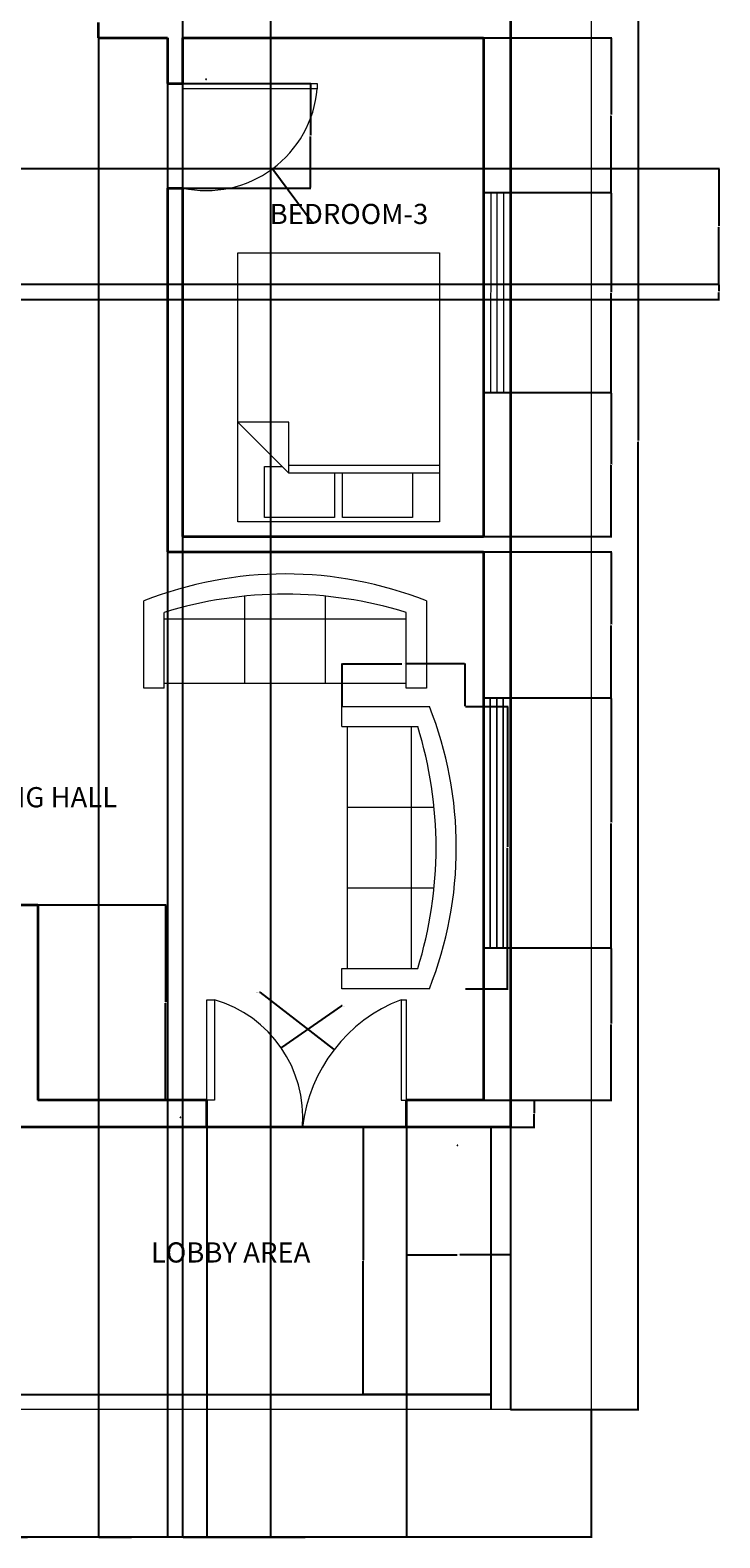
# Model space of a CAD drawing. Units: inches. Extents: x 4700 to 5209, y 8078 to 8754.
# Tile 3 of 5: x 5004 to 5209, y 8078 to 8526. Entities that reach past the tile are written whole.
import ezdxf

# ---------------------------------------------------------------- set-up
doc = ezdxf.new("R2010")
doc.units = ezdxf.units.IN
for name, color, linetype, lineweight in [('A-ANNO-DIMS', 2, 'Continuous', 18), ('A-AREA-IDEN', 7, 'Continuous', 18), ('A-DOOR', 3, 'Continuous', 18), ('A-FLOR', 7, 'Continuous', 25), ('A-FURN', 8, 'Continuous', 18), ('A-GLAZ', 4, 'Continuous', 18), ('A-WALL', 7, 'Continuous', 35), ('C-PROP', 8, 'Continuous', 18)]:
    doc.layers.add(name, color=color, linetype=linetype, lineweight=lineweight)
doc.styles.get("Standard").update_dxf_attribs({"font": 'arial.ttf'})
doc.dimstyles.get("Standard").update_dxf_attribs({"dimtxt": 0.18, "dimasz": 0.18, "dimexe": 0.18, "dimexo": 0.0625, "dimgap": 0.09, "dimtad": 0, "dimtih": 1, "dimtoh": 1, "dimdec": 4, "dimzin": 0, "dimdsep": 46, "dimtxsty": 'Standard', "dimcen": 0.09, "dimadec": 0, "dimazin": 0, "dimtfac": 1, "dimtdec": 4, "dimtofl": 0, "dimtmove": 0, "dimatfit": 3, "dimfxl": 1, "dimtolj": 1, "dimtzin": 0, "dimarcsym": 0})

# ---------------------------------------------------------------- blocks, each defined once
blk = doc.blocks.new('Sofa - Roundback 7 ft.')
for p, q in [((-12.00002, -32.4421), (-12.00003, -6.5971)), ((11.99997, -32.4421), (11.99998, -6.5971)), ((-36.000027, -34), (-36.000027, -11.4696)), ((-35.999844, -13.3819), (35.9998, -13.3819)), ((35.99998, -34), (35.99998, -11.4696)), ((-36.000027, -32.4421), (35.99998, -32.4421))]:
    blk.add_line(p, q)
for points in [[(-36.000027, -34), (-42.000027, -34), (-42.000027, -8)], [(41.99998, -8), (41.99998, -34), (35.99998, -34)]]:
    blk.add_lwpolyline(points)
for centre, radius, start, end in [((0, -114.25), 114.25, 68.43141, 111.5686), ((-0.00001, -127.1968), 121.1968, 72.72033, 107.2797)]:
    blk.add_arc(centre, radius, start, end)
blk = doc.blocks.new('Bed - Queen')
for p, q in [((0, -80.00003), (0, 0)), ((0, 0), (59.99999, 0)), ((59.99999, 0), (59.99999, -80.00003)), ((7.99999, -1.2), (28.79998, -1.2)), ((7.99999, -14.4), (7.99999, -1.2)), ((28.79998, -1.2), (28.79998, -14.4)), ((31.19999, -1.2), (51.99999, -1.2)), ((31.19999, -14.4), (31.19999, -1.2)), ((51.99999, -1.2), (51.99999, -16.4)), ((0, -14.4), (44.8, -14.4)), ((44.8, -16.8), (0, -16.8)), ((59.99999, -29.6), (44.8, -14.4)), ((44.8, -14.4), (44.8, -29.6)), ((51.99999, -16.4), (46.79936, -16.4)), ((44.8, -29.6), (59.99999, -29.6)), ((59.99999, -80.00003), (0, -80.00003))]:
    blk.add_line(p, q)
blk = doc.blocks.new('*D10')
at = {"layer": 'A-ANNO-DIMS', "color": 0, "lineweight": -2, "transparency": 16777216}
for p, q in [((5133.42, 8324.88), (5146.13, 8324.88)), ((5145.95, 8324.7), (5145.95, 8283.06)), ((5145.95, 8241.06), (5145.95, 8282.7)), ((5133.42, 8240.88), (5146.13, 8240.88))]:
    blk.add_line(p, q, dxfattribs=at)
at = {"layer": 'A-ANNO-DIMS', "color": 0, "transparency": 16777216}
for points in [[(5145.92, 8324.7), (5145.98, 8324.7), (5145.95, 8324.88)], [(5145.92, 8241.06), (5145.98, 8241.06), (5145.95, 8240.88)]]:
    blk.add_solid(points, dxfattribs=at)
at = {"layer": 'Defpoints', "color": 0, "transparency": 16777216}
for p in [(5133.35, 8324.88), (5133.35, 8240.88), (5145.95, 8240.88)]:
    blk.add_point(p, dxfattribs=at)
at = {"layer": 'A-ANNO-DIMS', "color": 0, "transparency": 16777216, "insert": (5145.95, 8282.88), "char_height": 0.18, "attachment_point": 5}
blk.add_mtext('\\A1;SOFA 84 TYP.', dxfattribs=at)
blk = doc.blocks.new('*D11')
at = {"layer": 'A-ANNO-DIMS', "color": 0, "lineweight": -2, "transparency": 16777216}
for p, q in [((5096.69, 8324.94), (5096.69, 8337.66)), ((5096.87, 8337.48), (5114.49, 8337.48)), ((5133.17, 8337.48), (5115.55, 8337.48)), ((5133.35, 8324.94), (5133.35, 8337.66))]:
    blk.add_line(p, q, dxfattribs=at)
at = {"layer": 'A-ANNO-DIMS', "color": 0, "transparency": 16777216}
for points in [[(5096.87, 8337.51), (5096.87, 8337.45), (5096.69, 8337.48)], [(5133.17, 8337.51), (5133.17, 8337.45), (5133.35, 8337.48)]]:
    blk.add_solid(points, dxfattribs=at)
at = {"layer": 'Defpoints', "color": 0, "transparency": 16777216}
for p in [(5133.35, 8337.48), (5096.69, 8324.88), (5133.35, 8324.88)]:
    blk.add_point(p, dxfattribs=at)
at = {"layer": 'A-ANNO-DIMS', "color": 0, "transparency": 16777216, "insert": (5115.02, 8337.48), "char_height": 0.18, "attachment_point": 5}
blk.add_mtext('\\A1;37 TYP.', dxfattribs=at)
blk = doc.blocks.new('*D14')
at = {"layer": 'A-ANNO-DIMS', "color": 0, "lineweight": -2, "transparency": 16777216}
for p, q in [((4738.78, 8115.69), (4738.78, 8077.57)), ((5170.78, 8115.69), (5170.78, 8077.57)), ((4738.96, 8077.75), (4954.49, 8077.75)), ((5170.6, 8077.75), (4955.07, 8077.75))]:
    blk.add_line(p, q, dxfattribs=at)
at = {"layer": 'A-ANNO-DIMS', "color": 0, "transparency": 16777216}
for points in [[(4738.96, 8077.78), (4738.96, 8077.72), (4738.78, 8077.75)], [(5170.6, 8077.78), (5170.6, 8077.72), (5170.78, 8077.75)]]:
    blk.add_solid(points, dxfattribs=at)
at = {"layer": 'Defpoints', "color": 0, "transparency": 16777216}
for p in [(4738.78, 8115.75), (5170.78, 8115.75), (5170.78, 8077.75)]:
    blk.add_point(p, dxfattribs=at)
at = {"layer": 'A-ANNO-DIMS', "color": 0, "transparency": 16777216, "insert": (4954.78, 8077.75), "char_height": 0.18, "attachment_point": 5}
blk.add_mtext('\\A1;432', dxfattribs=at)
blk = doc.blocks.new('*D17')
at = {"layer": 'A-ANNO-DIMS', "color": 0, "lineweight": -2, "transparency": 16777216}
for p, q in [((5146.84, 8691.75), (5184.96, 8691.75)), ((5184.78, 8691.57), (5184.78, 8403.93)), ((5184.78, 8115.93), (5184.78, 8403.57)), ((5146.84, 8115.75), (5184.96, 8115.75))]:
    blk.add_line(p, q, dxfattribs=at)
at = {"layer": 'A-ANNO-DIMS', "color": 0, "transparency": 16777216}
for points in [[(5184.75, 8691.57), (5184.81, 8691.57), (5184.78, 8691.75)], [(5184.75, 8115.93), (5184.81, 8115.93), (5184.78, 8115.75)]]:
    blk.add_solid(points, dxfattribs=at)
at = {"layer": 'Defpoints', "color": 0, "transparency": 16777216}
for p in [(5146.78, 8691.75), (5146.78, 8115.75), (5184.78, 8115.75)]:
    blk.add_point(p, dxfattribs=at)
at = {"layer": 'A-ANNO-DIMS', "color": 0, "transparency": 16777216, "insert": (5184.78, 8403.75), "char_height": 0.18, "attachment_point": 5}
blk.add_mtext('\\A1;576', dxfattribs=at)
blk = doc.blocks.new('*D38')
at = {"layer": 'A-ANNO-DIMS', "color": 0, "lineweight": -2, "transparency": 16777216}
for p, q in [((5138.84, 8253.05), (5176.96, 8253.05)), ((5176.78, 8252.87), (5176.78, 8230.58)), ((5176.78, 8207.93), (5176.78, 8230.22)), ((5138.84, 8207.75), (5176.96, 8207.75))]:
    blk.add_line(p, q, dxfattribs=at)
at = {"layer": 'A-ANNO-DIMS', "color": 0, "transparency": 16777216}
for points in [[(5176.75, 8252.87), (5176.81, 8252.87), (5176.78, 8253.05)], [(5176.75, 8207.93), (5176.81, 8207.93), (5176.78, 8207.75)]]:
    blk.add_solid(points, dxfattribs=at)
at = {"layer": 'Defpoints', "color": 0, "transparency": 16777216}
for p in [(5138.78, 8253.05), (5138.78, 8207.75), (5176.78, 8207.75)]:
    blk.add_point(p, dxfattribs=at)
at = {"layer": 'A-ANNO-DIMS', "color": 0, "transparency": 16777216, "insert": (5176.78, 8230.4), "char_height": 0.18, "attachment_point": 5}
blk.add_mtext('\\A1;45.3', dxfattribs=at)
blk = doc.blocks.new('*D39')
at = {"layer": 'A-ANNO-DIMS', "color": 0, "lineweight": -2, "transparency": 16777216}
for p, q in [((5138.84, 8327.41), (5176.96, 8327.41)), ((5176.78, 8327.23), (5176.78, 8290.41)), ((5176.78, 8253.23), (5176.78, 8290.05)), ((5138.84, 8253.05), (5176.96, 8253.05))]:
    blk.add_line(p, q, dxfattribs=at)
at = {"layer": 'A-ANNO-DIMS', "color": 0, "transparency": 16777216}
for points in [[(5176.75, 8327.23), (5176.81, 8327.23), (5176.78, 8327.41)], [(5176.75, 8253.23), (5176.81, 8253.23), (5176.78, 8253.05)]]:
    blk.add_solid(points, dxfattribs=at)
at = {"layer": 'Defpoints', "color": 0, "transparency": 16777216}
for p in [(5138.78, 8327.41), (5138.78, 8253.05), (5176.78, 8253.05)]:
    blk.add_point(p, dxfattribs=at)
at = {"layer": 'A-ANNO-DIMS', "color": 0, "transparency": 16777216, "insert": (5176.78, 8290.23), "char_height": 0.18, "attachment_point": 5}
blk.add_mtext('\\A1;74.36', dxfattribs=at)
blk = doc.blocks.new('*D40')
at = {"layer": 'A-ANNO-DIMS', "color": 0, "lineweight": -2, "transparency": 16777216}
for p, q in [((5138.84, 8370.85), (5176.96, 8370.85)), ((5176.78, 8370.67), (5176.78, 8349.31)), ((5176.78, 8327.59), (5176.78, 8348.95)), ((5138.84, 8327.41), (5176.96, 8327.41))]:
    blk.add_line(p, q, dxfattribs=at)
at = {"layer": 'A-ANNO-DIMS', "color": 0, "transparency": 16777216}
for points in [[(5176.75, 8370.67), (5176.81, 8370.67), (5176.78, 8370.85)], [(5176.75, 8327.59), (5176.81, 8327.59), (5176.78, 8327.41)]]:
    blk.add_solid(points, dxfattribs=at)
at = {"layer": 'Defpoints', "color": 0, "transparency": 16777216}
for p in [(5138.78, 8370.85), (5138.78, 8327.41), (5176.78, 8327.41)]:
    blk.add_point(p, dxfattribs=at)
at = {"layer": 'A-ANNO-DIMS', "color": 0, "transparency": 16777216, "insert": (5176.78, 8349.13), "char_height": 0.18, "attachment_point": 5}
blk.add_mtext('\\A1;43.44', dxfattribs=at)
blk = doc.blocks.new('*D41')
at = {"layer": 'A-ANNO-DIMS', "color": 0, "lineweight": -2, "transparency": 16777216}
for p, q in [((5138.84, 8418.18), (5176.96, 8418.18)), ((5176.78, 8418), (5176.78, 8396.95)), ((5176.78, 8375.53), (5176.78, 8396.58)), ((5138.84, 8375.35), (5176.96, 8375.35))]:
    blk.add_line(p, q, dxfattribs=at)
at = {"layer": 'A-ANNO-DIMS', "color": 0, "transparency": 16777216}
for points in [[(5176.75, 8418), (5176.81, 8418), (5176.78, 8418.18)], [(5176.75, 8375.53), (5176.81, 8375.53), (5176.78, 8375.35)]]:
    blk.add_solid(points, dxfattribs=at)
at = {"layer": 'Defpoints', "color": 0, "transparency": 16777216}
for p in [(5138.78, 8418.18), (5138.78, 8375.35), (5176.78, 8375.35)]:
    blk.add_point(p, dxfattribs=at)
at = {"layer": 'A-ANNO-DIMS', "color": 0, "transparency": 16777216, "insert": (5176.78, 8396.77), "char_height": 0.18, "attachment_point": 5}
blk.add_mtext('\\A1;42.83', dxfattribs=at)
blk = doc.blocks.new('*D42')
at = {"layer": 'A-ANNO-DIMS', "color": 0, "lineweight": -2, "transparency": 16777216}
for p, q in [((5138.84, 8477.68), (5176.96, 8477.68)), ((5176.78, 8477.5), (5176.78, 8448.11)), ((5176.78, 8418.36), (5176.78, 8447.75)), ((5138.84, 8418.18), (5176.96, 8418.18))]:
    blk.add_line(p, q, dxfattribs=at)
at = {"layer": 'A-ANNO-DIMS', "color": 0, "transparency": 16777216}
for points in [[(5176.75, 8477.5), (5176.81, 8477.5), (5176.78, 8477.68)], [(5176.75, 8418.36), (5176.81, 8418.36), (5176.78, 8418.18)]]:
    blk.add_solid(points, dxfattribs=at)
at = {"layer": 'Defpoints', "color": 0, "transparency": 16777216}
for p in [(5138.78, 8477.68), (5138.78, 8418.18), (5176.78, 8418.18)]:
    blk.add_point(p, dxfattribs=at)
at = {"layer": 'A-ANNO-DIMS', "color": 0, "transparency": 16777216, "insert": (5176.78, 8447.93), "char_height": 0.18, "attachment_point": 5}
blk.add_mtext('\\A1;59.5', dxfattribs=at)
blk = doc.blocks.new('*D43')
at = {"layer": 'A-ANNO-DIMS', "color": 0, "lineweight": -2, "transparency": 16777216}
for p, q in [((5138.84, 8523.75), (5176.96, 8523.75)), ((5176.78, 8523.57), (5176.78, 8500.9)), ((5176.78, 8477.86), (5176.78, 8500.53)), ((5138.84, 8477.68), (5176.96, 8477.68))]:
    blk.add_line(p, q, dxfattribs=at)
at = {"layer": 'A-ANNO-DIMS', "color": 0, "transparency": 16777216}
for points in [[(5176.75, 8523.57), (5176.81, 8523.57), (5176.78, 8523.75)], [(5176.75, 8477.86), (5176.81, 8477.86), (5176.78, 8477.68)]]:
    blk.add_solid(points, dxfattribs=at)
at = {"layer": 'Defpoints', "color": 0, "transparency": 16777216}
for p in [(5138.78, 8523.75), (5138.78, 8477.68), (5176.78, 8477.68)]:
    blk.add_point(p, dxfattribs=at)
at = {"layer": 'A-ANNO-DIMS', "color": 0, "transparency": 16777216, "insert": (5176.78, 8500.72), "char_height": 0.18, "attachment_point": 5}
blk.add_mtext('\\A1;46.07', dxfattribs=at)
blk = doc.blocks.new('*D48')
at = {"layer": 'A-ANNO-DIMS', "color": 0, "lineweight": -2, "transparency": 16777216}
for p, q in [((5140.92, 8199.75), (5102.8, 8199.75)), ((5102.98, 8199.57), (5102.98, 8160.18)), ((5102.98, 8120.43), (5102.98, 8159.82)), ((5140.92, 8120.25), (5102.8, 8120.25))]:
    blk.add_line(p, q, dxfattribs=at)
at = {"layer": 'A-ANNO-DIMS', "color": 0, "transparency": 16777216}
for points in [[(5102.95, 8199.57), (5103.01, 8199.57), (5102.98, 8199.75)], [(5102.95, 8120.43), (5103.01, 8120.43), (5102.98, 8120.25)]]:
    blk.add_solid(points, dxfattribs=at)
at = {"layer": 'Defpoints', "color": 0, "transparency": 16777216}
for p in [(5102.98, 8199.75), (5140.98, 8199.75), (5140.98, 8120.25)]:
    blk.add_point(p, dxfattribs=at)
at = {"layer": 'A-ANNO-DIMS', "color": 0, "transparency": 16777216, "insert": (5102.98, 8160), "char_height": 0.18, "attachment_point": 5}
blk.add_mtext('\\A1;79.5', dxfattribs=at)
blk = doc.blocks.new('*D56')
at = {"layer": 'A-ANNO-DIMS', "color": 0, "lineweight": -2, "transparency": 16777216}
for p, q in [((5006.24, 8265.86), (5044.35, 8265.86)), ((5044.17, 8265.68), (5044.17, 8236.99)), ((5044.17, 8207.93), (5044.17, 8236.62)), ((5006.24, 8207.75), (5044.35, 8207.75))]:
    blk.add_line(p, q, dxfattribs=at)
at = {"layer": 'A-ANNO-DIMS', "color": 0, "transparency": 16777216}
for points in [[(5044.14, 8265.68), (5044.2, 8265.68), (5044.17, 8265.86)], [(5044.14, 8207.93), (5044.2, 8207.93), (5044.17, 8207.75)]]:
    blk.add_solid(points, dxfattribs=at)
at = {"layer": 'Defpoints', "color": 0, "transparency": 16777216}
for p in [(5006.17, 8265.86), (5006.17, 8207.75), (5044.17, 8207.75)]:
    blk.add_point(p, dxfattribs=at)
at = {"layer": 'A-ANNO-DIMS', "color": 0, "transparency": 16777216, "insert": (5044.17, 8236.81), "char_height": 0.18, "attachment_point": 5}
blk.add_mtext('\\A1;58.11', dxfattribs=at)
blk = doc.blocks.new('*D57')
at = {"layer": 'A-ANNO-DIMS', "color": 0, "lineweight": -2, "transparency": 16777216}
for p, q in [((5056.45, 8199.69), (5056.45, 8077.57)), ((5115.89, 8199.69), (5115.89, 8077.57)), ((5056.63, 8077.75), (5085.78, 8077.75)), ((5115.71, 8077.75), (5086.57, 8077.75))]:
    blk.add_line(p, q, dxfattribs=at)
at = {"layer": 'A-ANNO-DIMS', "color": 0, "transparency": 16777216}
for points in [[(5056.63, 8077.78), (5056.63, 8077.72), (5056.45, 8077.75)], [(5115.71, 8077.78), (5115.71, 8077.72), (5115.89, 8077.75)]]:
    blk.add_solid(points, dxfattribs=at)
at = {"layer": 'Defpoints', "color": 0, "transparency": 16777216}
for p in [(5056.45, 8199.75), (5115.89, 8199.75), (5115.89, 8077.75)]:
    blk.add_point(p, dxfattribs=at)
at = {"layer": 'A-ANNO-DIMS', "color": 0, "transparency": 16777216, "insert": (5086.17, 8077.75), "char_height": 0.18, "attachment_point": 5}
blk.add_mtext('\\A1;59.44', dxfattribs=at)
blk = doc.blocks.new('*D58')
at = {"layer": 'A-ANNO-DIMS', "color": 0, "lineweight": -2, "transparency": 16777216}
for p, q in [((5115.89, 8199.69), (5115.89, 8161.57)), ((5146.78, 8199.69), (5146.78, 8161.57)), ((5116.07, 8161.75), (5130.94, 8161.75)), ((5146.6, 8161.75), (5131.73, 8161.75))]:
    blk.add_line(p, q, dxfattribs=at)
at = {"layer": 'A-ANNO-DIMS', "color": 0, "transparency": 16777216}
for points in [[(5116.07, 8161.78), (5116.07, 8161.72), (5115.89, 8161.75)], [(5146.6, 8161.78), (5146.6, 8161.72), (5146.78, 8161.75)]]:
    blk.add_solid(points, dxfattribs=at)
at = {"layer": 'Defpoints', "color": 0, "transparency": 16777216}
for p in [(5115.89, 8199.75), (5146.78, 8199.75), (5115.89, 8161.75)]:
    blk.add_point(p, dxfattribs=at)
at = {"layer": 'A-ANNO-DIMS', "color": 0, "transparency": 16777216, "insert": (5131.34, 8161.75), "char_height": 0.18, "attachment_point": 5}
blk.add_mtext('\\A1;30.89', dxfattribs=at)
blk = doc.blocks.new('*D64')
at = {"layer": 'A-ANNO-DIMS', "color": 0, "lineweight": -2, "transparency": 16777216}
for p, q in [((4982.78, 8523.69), (4982.78, 8077.57)), ((5024.22, 8523.69), (5024.22, 8077.57)), ((4982.96, 8077.75), (5003.1, 8077.75)), ((5024.04, 8077.75), (5003.9, 8077.75))]:
    blk.add_line(p, q, dxfattribs=at)
at = {"layer": 'A-ANNO-DIMS', "color": 0, "transparency": 16777216}
for points in [[(4982.96, 8077.78), (4982.96, 8077.72), (4982.78, 8077.75)], [(5024.04, 8077.78), (5024.04, 8077.72), (5024.22, 8077.75)]]:
    blk.add_solid(points, dxfattribs=at)
at = {"layer": 'Defpoints', "color": 0, "transparency": 16777216}
for p in [(4982.78, 8523.75), (5024.22, 8523.75), (5024.22, 8077.75)]:
    blk.add_point(p, dxfattribs=at)
at = {"layer": 'A-ANNO-DIMS', "color": 0, "transparency": 16777216, "insert": (5003.5, 8077.75), "char_height": 0.18, "attachment_point": 5}
blk.add_mtext('\\A1;41.44', dxfattribs=at)
blk = doc.blocks.new('*D66')
at = {"layer": 'A-ANNO-DIMS', "color": 0, "lineweight": -2, "transparency": 16777216}
for p, q in [((5024.22, 8523.69), (5024.22, 8077.57)), ((5044.78, 8523.69), (5044.78, 8077.57)), ((5024.4, 8077.75), (5034.1, 8077.75)), ((5044.6, 8077.75), (5034.89, 8077.75))]:
    blk.add_line(p, q, dxfattribs=at)
at = {"layer": 'A-ANNO-DIMS', "color": 0, "transparency": 16777216}
for points in [[(5024.4, 8077.78), (5024.4, 8077.72), (5024.22, 8077.75)], [(5044.6, 8077.78), (5044.6, 8077.72), (5044.78, 8077.75)]]:
    blk.add_solid(points, dxfattribs=at)
at = {"layer": 'Defpoints', "color": 0, "transparency": 16777216}
for p in [(5024.22, 8523.75), (5044.78, 8523.75), (5044.78, 8077.75)]:
    blk.add_point(p, dxfattribs=at)
at = {"layer": 'A-ANNO-DIMS', "color": 0, "transparency": 16777216, "insert": (5034.5, 8077.75), "char_height": 0.18, "attachment_point": 5}
blk.add_mtext('\\A1;20.56', dxfattribs=at)
blk = doc.blocks.new('*D69')
at = {"layer": 'A-ANNO-DIMS', "color": 0, "lineweight": -2, "transparency": 16777216}
for p, q in [((5049.34, 8510.09), (5087.46, 8510.09)), ((5087.28, 8509.91), (5087.28, 8494.75)), ((5087.28, 8479.22), (5087.28, 8494.38)), ((5049.34, 8479.04), (5087.46, 8479.04))]:
    blk.add_line(p, q, dxfattribs=at)
at = {"layer": 'A-ANNO-DIMS', "color": 0, "transparency": 16777216}
for points in [[(5087.25, 8509.91), (5087.31, 8509.91), (5087.28, 8510.09)], [(5087.25, 8479.22), (5087.31, 8479.22), (5087.28, 8479.04)]]:
    blk.add_solid(points, dxfattribs=at)
at = {"layer": 'Defpoints', "color": 0, "transparency": 16777216}
for p in [(5049.28, 8510.09), (5049.28, 8479.04), (5087.28, 8479.04)]:
    blk.add_point(p, dxfattribs=at)
at = {"layer": 'A-ANNO-DIMS', "color": 0, "transparency": 16777216, "insert": (5087.28, 8494.56), "char_height": 0.18, "attachment_point": 5}
blk.add_mtext('\\A1;31.06', dxfattribs=at)
blk = doc.blocks.new('*D70')
at = {"layer": 'A-ANNO-DIMS', "color": 0, "lineweight": -2, "transparency": 16777216}
for p, q in [((4867.58, 8484.83), (5208.96, 8484.83)), ((5208.78, 8484.65), (5208.78, 8467.8)), ((5208.78, 8450.59), (5208.78, 8467.43)), ((4867.58, 8450.41), (5208.96, 8450.41))]:
    blk.add_line(p, q, dxfattribs=at)
at = {"layer": 'A-ANNO-DIMS', "color": 0, "transparency": 16777216}
for points in [[(5208.75, 8484.65), (5208.81, 8484.65), (5208.78, 8484.83)], [(5208.75, 8450.59), (5208.81, 8450.59), (5208.78, 8450.41)]]:
    blk.add_solid(points, dxfattribs=at)
at = {"layer": 'Defpoints', "color": 0, "transparency": 16777216}
for p in [(4867.52, 8484.83), (5208.78, 8484.83), (4867.52, 8450.41)]:
    blk.add_point(p, dxfattribs=at)
at = {"layer": 'A-ANNO-DIMS', "color": 0, "transparency": 16777216, "insert": (5208.78, 8467.62), "char_height": 0.18, "attachment_point": 5}
blk.add_mtext('\\A1;34.42', dxfattribs=at)
blk = doc.blocks.new('*D71')
at = {"layer": 'A-ANNO-DIMS', "color": 0, "lineweight": -2, "transparency": 16777216}
for p, q in [((5049.28, 8647.34), (5049.28, 8077.57)), ((5075.44, 8647.34), (5075.44, 8077.57)), ((5049.46, 8077.75), (5061.97, 8077.75)), ((5075.26, 8077.75), (5062.76, 8077.75))]:
    blk.add_line(p, q, dxfattribs=at)
at = {"layer": 'A-ANNO-DIMS', "color": 0, "transparency": 16777216}
for points in [[(5049.46, 8077.78), (5049.46, 8077.72), (5049.28, 8077.75)], [(5075.26, 8077.78), (5075.26, 8077.72), (5075.44, 8077.75)]]:
    blk.add_solid(points, dxfattribs=at)
at = {"layer": 'Defpoints', "color": 0, "transparency": 16777216}
for p in [(5049.28, 8647.41), (5075.44, 8647.41), (5075.44, 8077.75)]:
    blk.add_point(p, dxfattribs=at)
at = {"layer": 'A-ANNO-DIMS', "color": 0, "transparency": 16777216, "insert": (5062.36, 8077.75), "char_height": 0.18, "attachment_point": 5}
blk.add_mtext('\\A1;26.16', dxfattribs=at)
blk = doc.blocks.new('*D75')
at = {"layer": 'A-ANNO-DIMS', "color": 0, "lineweight": -2, "transparency": 16777216}
for p, q in [((5115.95, 8207.75), (5154.07, 8207.75)), ((5153.89, 8207.57), (5153.89, 8203.93)), ((5153.89, 8199.93), (5153.89, 8203.57)), ((5115.95, 8199.75), (5154.07, 8199.75))]:
    blk.add_line(p, q, dxfattribs=at)
at = {"layer": 'A-ANNO-DIMS', "color": 0, "transparency": 16777216}
for points in [[(5153.86, 8207.57), (5153.92, 8207.57), (5153.89, 8207.75)], [(5153.86, 8199.93), (5153.92, 8199.93), (5153.89, 8199.75)]]:
    blk.add_solid(points, dxfattribs=at)
at = {"layer": 'Defpoints', "color": 0, "transparency": 16777216}
for p in [(5115.89, 8207.75), (5115.89, 8199.75), (5153.89, 8199.75)]:
    blk.add_point(p, dxfattribs=at)
at = {"layer": 'A-ANNO-DIMS', "color": 0, "transparency": 16777216, "insert": (5153.89, 8203.75), "char_height": 0.18, "attachment_point": 5}
blk.add_mtext('\\A1;8', dxfattribs=at)
blk = doc.blocks.new('*D76')
at = {"layer": 'A-ANNO-DIMS', "color": 0, "lineweight": -2, "transparency": 16777216}
for p, q in [((4867.58, 8450.41), (5208.96, 8450.41)), ((5208.78, 8450.23), (5208.78, 8448.34)), ((4867.58, 8445.91), (5208.96, 8445.91)), ((5208.78, 8446.09), (5208.78, 8447.97))]:
    blk.add_line(p, q, dxfattribs=at)
at = {"layer": 'A-ANNO-DIMS', "color": 0, "transparency": 16777216}
for points in [[(5208.75, 8450.23), (5208.81, 8450.23), (5208.78, 8450.41)], [(5208.75, 8446.09), (5208.81, 8446.09), (5208.78, 8445.91)]]:
    blk.add_solid(points, dxfattribs=at)
at = {"layer": 'Defpoints', "color": 0, "transparency": 16777216}
for p in [(4867.52, 8450.41), (4867.52, 8445.91), (5208.78, 8445.91)]:
    blk.add_point(p, dxfattribs=at)
at = {"layer": 'A-ANNO-DIMS', "color": 0, "transparency": 16777216, "insert": (5208.78, 8448.16), "char_height": 0.18, "attachment_point": 5}
blk.add_mtext('\\A1;4.5', dxfattribs=at)
blk = doc.blocks.new('*D77')
at = {"layer": 'A-ANNO-DIMS', "color": 0, "lineweight": -2, "transparency": 16777216}
for p, q in [((5072.1, 8239.84), (5072.28, 8239.84)), ((5072.28, 8239.84), (5094.19, 8222.88)), ((5130.99, 8194.32), (5131.17, 8194.32)), ((5131.08, 8194.23), (5131.08, 8194.41))]:
    blk.add_line(p, q, dxfattribs=at)
at = {"layer": 'A-ANNO-DIMS', "color": 0, "transparency": 16777216}
blk.add_solid([(5094.2, 8222.9), (5094.17, 8222.85), (5094.33, 8222.77)], dxfattribs=at)
at = {"layer": 'Defpoints', "color": 0, "transparency": 16777216}
for p in [(5094.33, 8222.77), (5131.08, 8194.32)]:
    blk.add_point(p, dxfattribs=at)
at = {"layer": 'A-ANNO-DIMS', "color": 0, "transparency": 16777216, "insert": (5071.62, 8239.84), "char_height": 0.18, "attachment_point": 5}
blk.add_mtext('\\A1;R46.47', dxfattribs=at)
blk = doc.blocks.new('*D78')
at = {"layer": 'A-ANNO-DIMS', "color": 0, "lineweight": -2, "transparency": 16777216}
for p, q in [((5096.55, 8235.79), (5078.72, 8223.46)), ((5096.73, 8235.79), (5096.55, 8235.79)), ((5048.53, 8202.65), (5048.71, 8202.65)), ((5048.62, 8202.56), (5048.62, 8202.74))]:
    blk.add_line(p, q, dxfattribs=at)
at = {"layer": 'A-ANNO-DIMS', "color": 0, "transparency": 16777216}
blk.add_solid([(5078.71, 8223.49), (5078.74, 8223.44), (5078.57, 8223.36)], dxfattribs=at)
at = {"layer": 'Defpoints', "color": 0, "transparency": 16777216}
for p in [(5078.57, 8223.36), (5048.62, 8202.65)]:
    blk.add_point(p, dxfattribs=at)
at = {"layer": 'A-ANNO-DIMS', "color": 0, "transparency": 16777216, "insert": (5097.21, 8235.79), "char_height": 0.18, "attachment_point": 5}
blk.add_mtext('\\A1;R36.42', dxfattribs=at)
blk = doc.blocks.new('*D81')
at = {"layer": 'A-ANNO-DIMS', "color": 0, "lineweight": -2, "transparency": 16777216}
for p, q in [((5056.22, 8511.41), (5056.4, 8511.41)), ((5056.31, 8511.32), (5056.31, 8511.5)), ((5087.78, 8468.75), (5076.08, 8484.6)), ((5087.96, 8468.75), (5087.78, 8468.75))]:
    blk.add_line(p, q, dxfattribs=at)
at = {"layer": 'A-ANNO-DIMS', "color": 0, "transparency": 16777216}
blk.add_solid([(5076.11, 8484.62), (5076.06, 8484.59), (5075.98, 8484.75)], dxfattribs=at)
at = {"layer": 'Defpoints', "color": 0, "transparency": 16777216}
for p in [(5056.31, 8511.41), (5075.98, 8484.75)]:
    blk.add_point(p, dxfattribs=at)
at = {"layer": 'A-ANNO-DIMS', "color": 0, "transparency": 16777216, "insert": (5088.44, 8468.75), "char_height": 0.18, "attachment_point": 5}
blk.add_mtext('\\A1;R33.13', dxfattribs=at)

msp = doc.modelspace()

# ---------------------------------------------------------------- linework, layer by layer
at = {"layer": 'A-DOOR'}
for p, q in [((5049.2803, 8510.0929), (5089.321, 8510.0929)), ((5049.2803, 8508.5669), (5049.2803, 8510.0929)), ((5089.321, 8508.5669), (5049.2803, 8508.5669)), ((5089.321, 8510.0929), (5089.321, 8510.0929)), ((5089.321, 8510.0929), (5089.321, 8508.5669)), ((5056.452, 8207.7503), (5056.452, 8237.638)), ((5056.452, 8237.638), (5058.7265, 8237.638)), ((5058.7265, 8237.638), (5058.7265, 8207.7503)), ((5114.2534, 8237.638), (5114.2534, 8207.7503)), ((5114.2534, 8237.638), (5115.8923, 8237.638)), ((5115.8923, 8207.7503), (5115.8923, 8237.638)), ((5058.7265, 8207.7503), (5056.452, 8207.7503)), ((5114.2534, 8207.7503), (5115.8923, 8207.7503))]:
    msp.add_line(p, q, dxfattribs=at)
for centre, radius, start, end in [((5056.3125, 8511.4116), 33.1309, 257.745546, 355.074383), ((5048.6169, 8202.6495), 36.4198, 355.434191, 73.883887), ((5131.0758, 8194.316), 46.4735, 111.221732, 173.284842)]:
    msp.add_arc(centre, radius, start, end, dxfattribs=at)
at = {"layer": 'A-FLOR'}
for p, q in [((5140.9801, 8199.7503), (5140.9801, 8115.7503)), ((5146.7803, 8199.7503), (5146.7803, 8115.7503)), ((4954.7803, 8120.2503), (5140.9801, 8120.2503))]:
    msp.add_line(p, q, dxfattribs=at)
at = {"layer": 'A-GLAZ'}
for p, q in [((5140.9494, 8477.6803), (5140.8581, 8418.1812)), ((5142.7803, 8477.6803), (5142.7803, 8418.1812)), ((5144.7137, 8477.6803), (5144.7731, 8418.1812))]:
    msp.add_line(p, q, dxfattribs=at)
for points in [[(5138.7803, 8477.6803), (5146.7803, 8477.6803), (5146.7803, 8418.1812), (5138.7803, 8418.1812)], [(5138.7803, 8327.4128), (5146.7803, 8327.4128), (5146.7803, 8253.0501), (5138.7803, 8253.0501)], [(5140.8015, 8327.4128), (5140.8015, 8327.4128), (5140.8015, 8253.0501), (5140.8015, 8253.0501)], [(5142.7803, 8327.4128), (5142.7803, 8327.4128), (5142.7803, 8253.0501), (5142.7803, 8253.0501)], [(5144.6769, 8327.4128), (5144.6769, 8327.4128), (5144.6769, 8253.0501), (5144.6769, 8253.0501)]]:
    msp.add_lwpolyline(points, close=True, dxfattribs=at)
at = {"layer": 'A-WALL'}
for p, q in [((5146.7803, 8691.7503), (5146.7803, 8199.7503)), ((5024.2192, 8523.7503), (5024.2192, 8528.2503)), ((5024.2192, 8523.7503), (5044.7803, 8523.7503)), ((5044.7803, 8523.7503), (5044.7803, 8510.0929)), ((5049.2803, 8523.7503), (5049.2803, 8510.0929)), ((5049.2803, 8523.7503), (5138.7803, 8523.7503)), ((5138.7803, 8523.7503), (5138.7803, 8375.3496)), ((5044.7803, 8510.0929), (5049.2803, 8510.0929)), ((5044.7803, 8479.0356), (5049.2803, 8479.0356)), ((5044.7803, 8479.0356), (5044.7803, 8370.8496)), ((5049.2803, 8479.0356), (5049.2803, 8375.3496)), ((5049.2803, 8375.3496), (5138.7803, 8375.3496)), ((5044.7803, 8370.8496), (5138.7803, 8370.8496)), ((5138.7803, 8370.8496), (5138.7803, 8207.7503)), ((4937.1464, 8265.8608), (5006.1744, 8265.8608)), ((5006.1744, 8265.8608), (5006.1744, 8207.7503)), ((5056.452, 8207.7503), (5006.1744, 8207.7503)), ((5056.452, 8199.7503), (5056.452, 8207.7503)), ((5138.7803, 8207.7503), (5115.8923, 8207.7503)), ((5115.8923, 8199.7503), (5115.8923, 8207.7503)), ((5146.7803, 8199.7503), (4762.7803, 8199.7503))]:
    msp.add_line(p, q, dxfattribs=at)
at = {"layer": 'C-PROP'}
for p, q in [((5170.7803, 8715.7503), (5170.7803, 8115.7503)), ((5170.7803, 8115.7503), (4738.7803, 8115.7503))]:
    msp.add_line(p, q, dxfattribs=at)

# ---------------------------------------------------------------- block references
at = {"layer": 'A-FURN'}
for name, p, rotation in [('Bed - Queen', (5125.6739, 8379.8105), 180), ('Sofa - Roundback 7 ft.', (5130.6879, 8282.8814), 270)]:
    msp.add_blockref(name, p, dxfattribs=dict(at, rotation=rotation))
msp.add_blockref('Sofa - Roundback 7 ft.', (5079.7803, 8364.2525), dxfattribs=at)

# ---------------------------------------------------------------- texts
at = {"layer": 'A-AREA-IDEN', "char_height": 6, "attachment_point": 1}
for s, width, insert in [('\\pxi-3,l4,t4;BEDROOM-3', 51.756341, (5069.1639, 8474.3356)), ('\\pxi-3,l4,t4;LIVING HALL ', 80.039779, (4976.653, 8300.8555)), ('LOBBY AREA', 78.457065, (5039.8534, 8165.4565))]:
    msp.add_mtext_dynamic_manual_height_columns(s, width=width, gutter_width=12.5, heights=[0], dxfattribs=dict(at, insert=insert))

# ---------------------------------------------------------------- dimensions: what is measured, and where the dimension line sits
at = {"layer": 'A-ANNO-DIMS'}
for base, p1, p2, angle, override, picture, middle in [((5184.7803, 8115.7503), (5146.7803, 8691.7503), (5146.7803, 8115.7503), 270, {"dimdec": 0, "dimlfac": 1, "dimrnd": 0, "dimzin": 0, "dimdsep": 46, "dimlunit": 2}, '*D17', (5184.7803, 8403.7503)), ((5176.7803, 8477.6803), (5138.7803, 8523.7503), (5138.7803, 8477.6803), 270, {"dimdec": 2, "dimlfac": 1, "dimrnd": 0, "dimzin": 0, "dimdsep": 46, "dimlunit": 2}, '*D43', (5176.7803, 8500.7153)), ((5087.2803, 8479.0356), (5049.2803, 8510.0929), (5049.2803, 8479.0356), 270, {"dimdec": 2, "dimlfac": 1, "dimrnd": 0, "dimzin": 0, "dimdsep": 46, "dimlunit": 2}, '*D69', (5087.2803, 8494.5643)), ((5208.7803, 8484.828), (4867.5173, 8450.4056), (4867.5173, 8484.828), 90, {"dimdec": 2, "dimlfac": 1, "dimrnd": 0, "dimzin": 0, "dimdsep": 46, "dimlunit": 2}, '*D70', (5208.7803, 8467.6168)), ((5176.7803, 8418.1812), (5138.7803, 8477.6803), (5138.7803, 8418.1812), 270, {"dimdec": 1, "dimlfac": 1, "dimrnd": 0, "dimzin": 0, "dimdsep": 46, "dimlunit": 2}, '*D42', (5176.7803, 8447.9308)), ((5208.7803, 8445.9056), (4867.5173, 8450.4056), (4867.5173, 8445.9056), 90, {"dimdec": 1, "dimlfac": 1, "dimrnd": 0, "dimzin": 0, "dimdsep": 46, "dimlunit": 2}, '*D76', (5208.7803, 8448.1556)), ((5176.7803, 8375.3496), (5138.7803, 8418.1812), (5138.7803, 8375.3496), 270, {"dimdec": 2, "dimlfac": 1, "dimrnd": 0, "dimzin": 0, "dimdsep": 46, "dimlunit": 2}, '*D41', (5176.7803, 8396.7654)), ((5176.7803, 8327.4128), (5138.7803, 8370.8496), (5138.7803, 8327.4128), 270, {"dimdec": 2, "dimlfac": 1, "dimrnd": 0, "dimzin": 0, "dimdsep": 46, "dimlunit": 2}, '*D40', (5176.7803, 8349.1312)), ((5176.7803, 8253.0501), (5138.7803, 8327.4128), (5138.7803, 8253.0501), 270, {"dimdec": 2, "dimlfac": 1, "dimrnd": 0, "dimzin": 0, "dimdsep": 46, "dimlunit": 2}, '*D39', (5176.7803, 8290.2314)), ((5044.1744, 8207.7503), (5006.1744, 8265.8608), (5006.1744, 8207.7503), 270, {"dimdec": 2, "dimlfac": 1, "dimrnd": 0, "dimzin": 0, "dimdsep": 46, "dimlunit": 2}, '*D56', (5044.1744, 8236.8056)), ((5176.7803, 8207.7503), (5138.7803, 8253.0501), (5138.7803, 8207.7503), 270, {"dimdec": 1, "dimlfac": 1, "dimrnd": 0, "dimzin": 0, "dimdsep": 46, "dimlunit": 2}, '*D38', (5176.7803, 8230.4002)), ((5153.8923, 8199.7503), (5115.8923, 8207.7503), (5115.8923, 8199.7503), 270, {"dimdec": 0, "dimlfac": 1, "dimrnd": 0, "dimzin": 0, "dimdsep": 46, "dimlunit": 2}, '*D75', (5153.8923, 8203.7503)), ((5102.9801, 8199.7503), (5140.9801, 8120.2503), (5140.9801, 8199.7503), 90, {"dimdec": 1, "dimlfac": 1, "dimrnd": 0, "dimzin": 0, "dimdsep": 46, "dimlunit": 2}, '*D48', (5102.9801, 8160.0003)), ((5115.8923, 8161.7503), (5146.7803, 8199.7503), (5115.8923, 8199.7503), 180, {"dimdec": 2, "dimlfac": 1, "dimrnd": 0, "dimzin": 0, "dimdsep": 46, "dimlunit": 2}, '*D58', (5131.3363, 8161.7503))]:
    dim = msp.add_linear_dim(base=base, p1=p1, p2=p2, angle=angle, dimstyle='Standard', override=override, dxfattribs=at)
    dim.commit()
    dim.dimension.update_dxf_attribs({"geometry": picture, "text_midpoint": middle})
for base, p1, p2, override, picture, middle in [((5075.4408, 8077.7503), (5049.2803, 8647.4059), (5075.4408, 8647.4059), {"dimdec": 2, "dimlfac": 1, "dimrnd": 0, "dimzin": 0, "dimdsep": 46, "dimlunit": 2}, '*D71', (5062.3606, 8077.7503)), ((5024.2192, 8077.7503), (4982.778, 8523.7503), (5024.2192, 8523.7503), {"dimdec": 2, "dimlfac": 1, "dimrnd": 0, "dimzin": 0, "dimdsep": 46, "dimlunit": 2}, '*D64', (5003.4986, 8077.7503)), ((5044.7803, 8077.7503), (5024.2192, 8523.7503), (5044.7803, 8523.7503), {"dimdec": 2, "dimlfac": 1, "dimrnd": 0, "dimzin": 0, "dimdsep": 46, "dimlunit": 2}, '*D66', (5034.4997, 8077.7503)), ((5115.8923, 8077.7503), (5056.452, 8199.7503), (5115.8923, 8199.7503), {"dimdec": 2, "dimlfac": 1, "dimrnd": 0, "dimzin": 0, "dimdsep": 46, "dimlunit": 2}, '*D57', (5086.1722, 8077.7503)), ((5170.7803, 8077.7503), (4738.7803, 8115.7503), (5170.7803, 8115.7503), {"dimdec": 0, "dimlfac": 1, "dimrnd": 0, "dimzin": 0, "dimdsep": 46, "dimlunit": 2}, '*D14', (4954.7803, 8077.7503))]:
    dim = msp.add_linear_dim(base=base, p1=p1, p2=p2, dimstyle='Standard', override=override, dxfattribs=at)
    dim.commit()
    dim.dimension.update_dxf_attribs({"geometry": picture, "text_midpoint": middle})
for center, mpoint, picture, middle in [((5056.3125, 8511.4116), (5075.9778, 8484.7483), '*D81', (5088.4368, 8468.7503)), ((5131.0758, 8194.316), (5094.3281, 8222.7659), '*D77', (5071.6197, 8239.8358)), ((5048.6169, 8202.6495), (5078.5741, 8223.3611), '*D78', (5097.2073, 8235.788))]:
    dim = msp.add_radius_dim(center=center, mpoint=mpoint, dimstyle='Standard', override={"dimdec": 2, "dimlfac": 1, "dimrnd": 0, "dimzin": 0, "dimdsep": 46, "dimlunit": 2}, dxfattribs=at)
    dim.commit()
    dim.dimension.update_dxf_attribs({"geometry": picture, "text_midpoint": middle, "dimtype": 164})
dim = msp.add_linear_dim(base=(5133.3546, 8337.4814), p1=(5096.6879, 8324.8814), p2=(5133.3546, 8324.8814), text='<> TYP.', dimstyle='Standard', override={"dimdec": 0, "dimlfac": 1, "dimrnd": 0, "dimzin": 0, "dimdsep": 46, "dimlunit": 2}, dxfattribs=at)
dim.commit()
dim.dimension.update_dxf_attribs({"geometry": '*D11', "text_midpoint": (5115.0212, 8337.4814)})
dim = msp.add_linear_dim(base=(5145.9546, 8240.8814), p1=(5133.3546, 8324.8814), p2=(5133.3546, 8240.8814), angle=270, text='SOFA <> TYP.', dimstyle='Standard', override={"dimdec": 0, "dimlfac": 1, "dimrnd": 0, "dimzin": 0, "dimdsep": 46, "dimlunit": 2}, dxfattribs=at)
dim.commit()
dim.dimension.update_dxf_attribs({"geometry": '*D10', "text_midpoint": (5145.9546, 8282.8814)})

doc.saveas('drawing.dxf')
